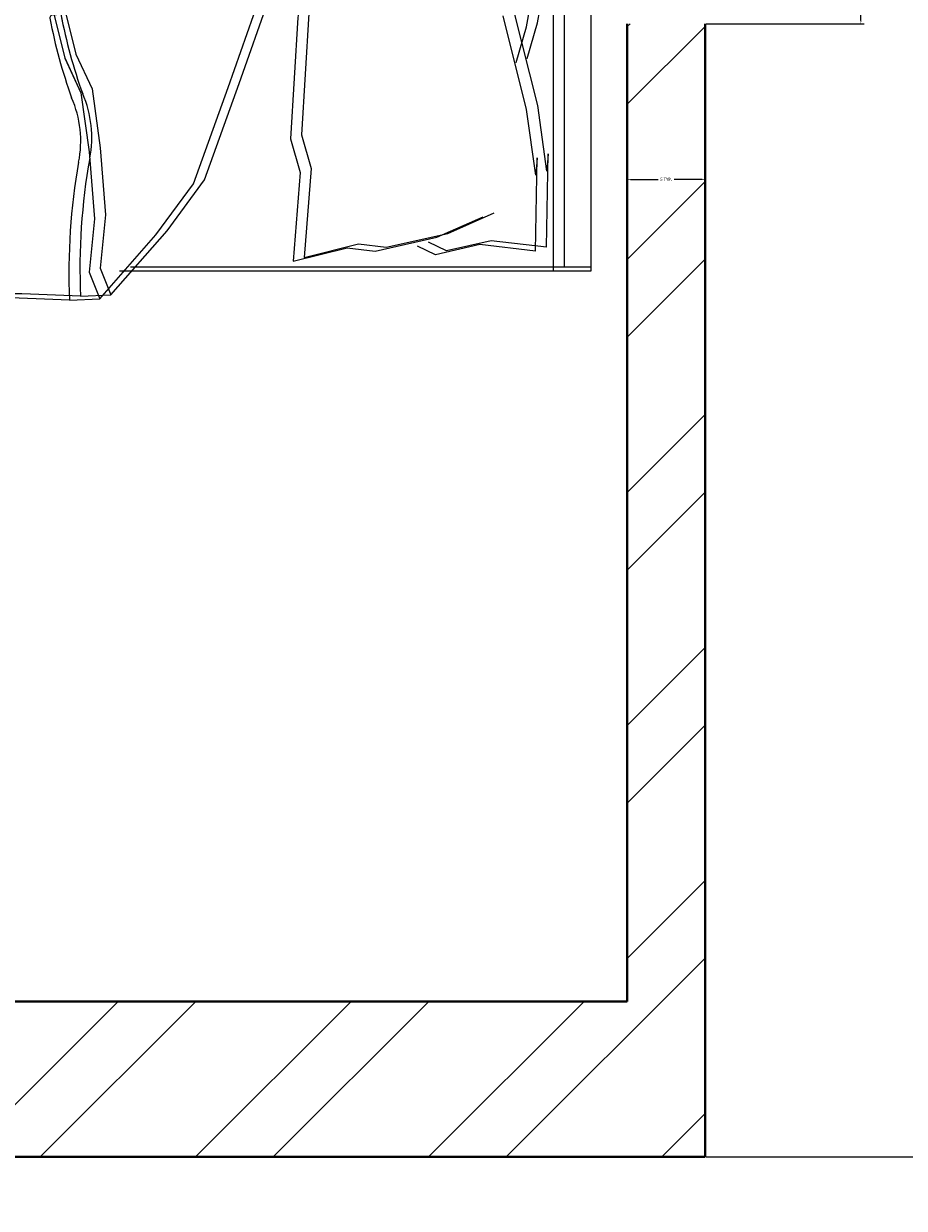
# Model space of a CAD drawing. Units: inches. Extents: x 1601 to 2297, y 1496 to 2631.
# Tile 19 of 57: x 2191 to 2242, y 1632 to 1701. Entities that reach past the tile are written whole.
import ezdxf

# ---------------------------------------------------------------- set-up
doc = ezdxf.new("R2010")
doc.units = ezdxf.units.IN
for name, color, linetype, lineweight in [('A-ANNO-DIMS', 2, 'Continuous', 18), ('A-FURN', 8, 'Continuous', 18), ('A-WALL', 7, 'Continuous', 40), ('A-WALL-PATT', 215, 'Continuous', 13)]:
    doc.layers.add(name, color=color, linetype=linetype, lineweight=lineweight)
doc.styles.get("Standard").update_dxf_attribs({"font": 'arial.ttf'})
doc.dimstyles.get("Standard").update_dxf_attribs({"dimtxt": 0.18, "dimasz": 0.18, "dimexe": 0.18, "dimexo": 0.0625, "dimgap": 0.09, "dimtad": 0, "dimtih": 1, "dimtoh": 1, "dimdec": 4, "dimzin": 0, "dimdsep": 46, "dimtxsty": 'Standard', "dimcen": 0.09, "dimadec": 0, "dimazin": 0, "dimtfac": 1, "dimtdec": 4, "dimtofl": 0, "dimtmove": 0, "dimatfit": 3, "dimfxl": 1, "dimtolj": 1, "dimtzin": 0, "dimarcsym": 0})

# ---------------------------------------------------------------- blocks, each defined once
blk = doc.blocks.new('BED-DOUBLE')
for p, q in [((27.746, 52.867), (24.495, 49.162)), ((27.746, 52.867), (24.495, 49.162)), ((27.746, 52.867), (24.495, 49.162)), ((27.746, 52.867), (24.495, 49.162)), ((28.385, 53.096), (25.135, 49.39)), ((28.385, 53.096), (25.135, 49.39)), ((28.385, 53.096), (25.135, 49.39)), ((28.385, 53.096), (25.135, 49.39)), ((29.49, 52.947), (27.746, 52.867, 3.871)), ((29.49, 52.947), (27.746, 52.867, 3.871)), ((29.49, 52.947), (27.746, 52.867, 3.871)), ((29.49, 52.947), (27.746, 52.867, 3.871)), ((28.365, 51.33), (27.746, 52.867)), ((28.365, 51.33), (27.746, 52.867)), ((28.365, 51.33), (27.746, 52.867)), ((28.365, 51.33), (27.746, 52.867)), ((30.13, 53.175), (28.385, 53.096, 3.871)), ((30.13, 53.175), (28.385, 53.096, 3.871)), ((30.13, 53.175), (28.385, 53.096, 3.871)), ((30.13, 53.175), (28.385, 53.096, 3.871)), ((29.004, 51.559), (28.385, 53.096)), ((29.004, 51.558), (28.385, 53.096)), ((29.004, 51.559), (28.385, 53.096)), ((29.004, 51.558), (28.385, 53.096)), ((0, 51.494), (0.639, 51.493)), ((0, 3.475), (0, 51.494)), ((0, 51.494), (0.639, 51.493)), ((0, 3.475), (0, 51.494)), ((0.639, 51.494), (27.249, 51.494)), ((0.639, 51.494), (27.249, 51.494)), ((0.639, 51.493), (27.249, 51.493)), ((0.639, 51.493), (27.249, 51.493)), ((2.173, 3.703), (2.173, 51.494)), ((2.173, 3.703), (2.173, 51.494)), ((2.173, 3.703), (2.173, 51.493)), ((2.173, 3.703), (2.173, 51.493)), ((28.695, 48.461), (29.004, 51.559)), ((28.695, 48.461), (29.004, 51.559)), ((28.695, 48.461), (29.004, 51.558)), ((28.695, 48.461), (29.004, 51.558)), ((0, 51.265), (26.61, 51.265)), ((0, 51.265), (26.61, 51.265)), ((0, 51.265), (26.61, 51.265)), ((0, 51.265), (26.61, 51.265)), ((1.533, 3.475), (1.533, 51.265)), ((1.533, 3.475), (1.533, 51.265)), ((1.533, 3.475), (1.533, 51.265)), ((1.533, 3.475), (1.533, 51.265)), ((16.573, 50.698), (13.434, 49.923)), ((16.573, 50.698), (13.434, 49.922)), ((16.573, 50.698), (13.434, 49.923)), ((16.573, 50.698), (13.434, 49.922)), ((17.212, 50.926), (14.073, 50.151)), ((17.212, 50.926), (14.073, 50.151)), ((17.212, 50.926), (14.073, 50.151)), ((17.212, 50.926), (14.073, 50.151)), ((16.169, 45.566), (16.573, 50.698)), ((16.169, 45.566), (16.573, 50.698)), ((16.169, 45.566), (16.573, 50.698)), ((16.169, 45.566), (16.573, 50.698)), ((16.808, 45.795), (17.212, 50.926)), ((16.808, 45.794), (17.212, 50.926)), ((16.808, 45.795), (17.212, 50.926)), ((16.808, 45.794), (17.212, 50.926)), ((28.055, 48.233), (28.365, 51.33)), ((28.055, 48.233), (28.365, 51.33)), ((28.055, 48.233), (28.365, 51.33)), ((28.055, 48.233), (28.365, 51.33)), ((2.557, 50.112), (2.46, 44.709)), ((2.557, 50.112), (2.46, 44.709)), ((2.557, 50.111), (2.46, 44.709)), ((2.557, 50.111), (2.46, 44.709)), ((2.557, 50.112), (5.768, 49.733)), ((2.557, 50.112), (5.768, 49.733)), ((2.557, 50.111), (5.768, 49.733)), ((2.557, 50.111), (5.768, 49.733)), ((3.196, 50.34), (3.099, 44.938)), ((3.196, 50.34), (3.099, 44.938)), ((3.196, 50.34), (3.099, 44.938)), ((3.196, 50.34), (3.099, 44.938)), ((3.196, 50.34), (6.407, 49.961)), ((3.196, 50.34), (6.407, 49.961)), ((3.196, 50.34), (6.407, 49.961)), ((3.196, 50.34), (6.407, 49.961)), ((5.768, 49.733), (8.338, 50.328)), ((5.768, 49.733), (8.338, 50.328)), ((5.768, 49.733), (8.338, 50.328)), ((5.768, 49.733), (8.338, 50.328)), ((6.407, 49.961), (8.977, 50.557)), ((6.407, 49.961), (8.977, 50.557)), ((6.407, 49.961), (8.977, 50.556)), ((6.407, 49.961), (8.977, 50.556)), ((11.829, 50.112), (8.257, 49.309)), ((11.829, 50.112), (8.257, 49.309)), ((11.829, 50.112), (8.257, 49.309)), ((11.829, 50.112), (8.257, 49.309)), ((8.338, 50.328), (9.384, 49.814)), ((8.338, 50.328), (9.384, 49.814)), ((8.338, 50.328), (9.384, 49.814)), ((8.338, 50.328), (9.384, 49.814)), ((12.468, 50.34), (8.896, 49.538)), ((12.468, 50.34), (8.896, 49.537)), ((12.468, 50.34), (8.896, 49.538)), ((12.468, 50.34), (8.896, 49.537)), ((8.977, 50.557), (10.024, 50.043)), ((8.977, 50.557), (10.024, 50.043)), ((8.977, 50.556), (10.024, 50.042)), ((8.977, 50.556), (10.024, 50.042)), ((13.434, 49.923), (11.829, 50.112)), ((13.434, 49.922), (11.829, 50.112)), ((13.434, 49.923), (11.829, 50.112)), ((13.434, 49.922), (11.829, 50.112)), ((14.073, 50.151), (12.468, 50.34)), ((14.073, 50.151), (12.468, 50.34)), ((14.073, 50.151), (12.468, 50.34)), ((14.073, 50.151), (12.468, 50.34)), ((8.896, 49.538), (6.218, 48.356)), ((8.896, 49.538), (6.218, 48.356)), ((8.896, 49.537), (6.218, 48.356)), ((8.896, 49.537), (6.218, 48.356)), ((25.135, 49.39), (22.968, 46.448)), ((25.135, 49.39), (22.968, 46.448)), ((25.135, 49.39), (22.968, 46.448)), ((25.135, 49.39), (22.968, 46.448)), ((8.257, 49.309), (5.578, 48.128)), ((8.257, 49.309), (5.578, 48.128)), ((8.257, 49.309), (5.578, 48.128)), ((8.257, 49.309), (5.578, 48.128)), ((24.495, 49.162), (22.329, 46.219)), ((24.495, 49.162), (22.329, 46.219)), ((24.495, 49.162), (22.329, 46.219)), ((24.495, 49.162), (22.329, 46.219)), ((28.365, 44.361), (28.055, 48.233)), ((28.365, 44.361), (28.055, 48.233)), ((28.365, 44.361), (28.055, 48.233)), ((28.365, 44.361), (28.055, 48.233)), ((29.004, 44.589), (28.695, 48.461)), ((29.004, 44.589), (28.695, 48.461)), ((29.004, 44.589), (28.695, 48.461)), ((29.004, 44.589), (28.695, 48.461)), ((3.099, 44.938), (3.181, 45.941)), ((3.099, 44.938), (3.181, 45.941)), ((3.099, 44.938), (3.181, 45.94)), ((3.099, 44.938), (3.181, 45.94)), ((3.181, 45.941), (3.709, 42.143)), ((3.181, 45.941), (3.709, 42.143)), ((3.181, 45.94), (3.709, 42.142)), ((3.181, 45.94), (3.709, 42.142)), ((22.329, 46.219), (20.316, 40.644)), ((22.329, 46.219), (20.316, 40.644)), ((22.329, 46.219), (20.317, 40.644)), ((22.329, 46.219), (20.317, 40.644)), ((22.968, 46.448), (20.956, 40.872)), ((22.968, 46.448), (20.956, 40.872)), ((22.968, 46.448), (20.956, 40.872)), ((22.968, 46.448), (20.956, 40.872)), ((2.46, 44.709), (2.542, 45.712)), ((2.46, 44.709), (2.542, 45.712)), ((2.46, 44.709), (2.542, 45.712)), ((2.46, 44.709), (2.542, 45.712)), ((2.542, 45.712), (3.069, 41.914)), ((2.542, 45.712), (3.069, 41.914)), ((2.542, 45.712), (3.069, 41.914)), ((2.542, 45.712), (3.069, 41.914)), ((16.726, 43.606), (16.169, 45.566)), ((16.726, 43.606), (16.169, 45.566)), ((16.726, 43.606), (16.169, 45.566)), ((16.726, 43.606), (16.169, 45.566)), ((17.365, 43.834), (16.808, 45.795)), ((17.365, 43.834), (16.808, 45.795)), ((17.365, 43.834), (16.808, 45.794)), ((17.365, 43.834), (16.808, 45.794)), ((29.468, 41.182), (29.004, 44.589)), ((29.469, 41.182), (29.004, 44.589)), ((29.468, 41.182), (29.004, 44.589)), ((29.469, 41.182), (29.004, 44.589)), ((28.829, 40.954), (28.365, 44.361)), ((28.829, 40.953), (28.365, 44.361)), ((28.829, 40.954), (28.365, 44.361)), ((28.829, 40.953), (28.365, 44.361)), ((16.295, 36.596), (16.726, 43.606)), ((16.295, 36.596), (16.726, 43.606)), ((16.295, 36.596), (16.726, 43.606)), ((16.295, 36.596), (16.726, 43.606)), ((16.934, 36.824), (17.365, 43.834)), ((16.934, 36.824), (17.365, 43.834)), ((16.934, 36.824), (17.365, 43.834)), ((16.934, 36.824), (17.365, 43.834)), ((3.069, 41.914), (4.422, 36.495)), ((3.069, 41.914), (4.422, 36.495)), ((3.069, 41.914), (4.422, 36.495)), ((3.069, 41.914), (4.422, 36.495)), ((3.709, 42.143), (5.061, 36.723)), ((3.709, 42.143), (5.061, 36.723)), ((3.709, 42.142), (5.061, 36.723)), ((3.709, 42.142), (5.061, 36.723)), ((30.397, 39.169), (29.468, 41.182)), ((30.397, 39.169), (29.468, 41.182)), ((30.397, 39.168), (29.469, 41.182)), ((30.397, 39.168), (29.469, 41.182)), ((20.316, 40.644), (17.383, 32.306)), ((20.317, 40.644), (17.383, 32.306)), ((20.316, 40.644), (17.383, 32.306)), ((20.317, 40.644), (17.383, 32.306)), ((20.956, 40.872), (18.022, 32.534)), ((20.956, 40.872), (18.022, 32.534)), ((20.956, 40.872), (18.022, 32.534)), ((20.956, 40.872), (18.022, 32.534)), ((29.758, 38.94), (28.829, 40.954)), ((29.758, 38.94), (28.829, 40.954)), ((29.758, 38.94), (28.829, 40.953)), ((29.758, 38.94), (28.829, 40.953)), ((79.884, 15.292), (79.884, 39.905)), ((79.884, 15.291), (79.884, 39.905)), ((79.884, 15.292), (79.884, 39.905)), ((79.884, 15.291), (79.884, 39.905)), ((3.673, 39.2), (3.078, 37.135)), ((3.673, 39.2), (3.078, 37.135)), ((3.673, 39.2), (3.078, 37.135)), ((3.673, 39.2), (3.078, 37.135)), ((4.313, 39.428), (3.717, 37.363)), ((4.313, 39.428), (3.717, 37.363)), ((4.313, 39.428), (3.718, 37.363)), ((4.313, 39.428), (3.718, 37.363)), ((31.016, 36.691), (30.397, 39.169)), ((31.016, 36.691), (30.397, 39.169)), ((31.016, 36.691), (30.397, 39.168)), ((31.016, 36.691), (30.397, 39.168)), ((79.245, 15.063), (79.245, 39.677)), ((79.245, 15.063), (79.245, 39.677)), ((79.245, 15.063), (79.245, 39.677)), ((79.245, 15.063), (79.245, 39.677)), ((30.377, 36.462), (29.758, 38.94)), ((30.377, 36.462), (29.758, 38.94)), ((30.377, 36.462), (29.758, 38.94)), ((30.377, 36.462), (29.758, 38.94)), ((3.078, 37.135), (2.537, 34.204)), ((3.078, 37.135), (2.537, 34.204)), ((3.078, 37.135), (2.537, 34.204)), ((3.078, 37.135), (2.537, 34.204)), ((3.717, 37.363), (3.176, 34.433)), ((3.718, 37.363), (3.176, 34.433)), ((3.717, 37.363), (3.176, 34.433)), ((3.718, 37.363), (3.176, 34.433)), ((15.628, 32.564), (16.295, 36.596)), ((15.628, 32.564), (16.295, 36.596)), ((15.628, 32.564), (16.295, 36.596)), ((15.628, 32.564), (16.295, 36.596)), ((16.268, 32.792), (16.934, 36.824)), ((16.268, 32.792), (16.934, 36.824)), ((16.268, 32.792), (16.934, 36.824)), ((16.268, 32.792), (16.934, 36.824)), ((24.516, 34.677), (29.004, 36.381)), ((24.516, 34.677), (29.004, 36.381)), ((24.516, 34.677), (29.004, 36.381)), ((24.516, 34.677), (29.004, 36.381)), ((28.365, 36.153), (30.377, 36.462)), ((28.365, 36.152), (30.377, 36.462)), ((28.365, 36.153), (30.377, 36.462)), ((28.365, 36.152), (30.377, 36.462)), ((29.004, 36.381), (31.016, 36.691)), ((29.004, 36.381), (31.016, 36.691)), ((29.004, 36.381), (31.016, 36.691)), ((29.004, 36.381), (31.016, 36.691)), ((23.876, 34.449), (28.365, 36.153)), ((23.876, 34.449), (28.365, 36.153)), ((23.876, 34.449), (28.365, 36.152)), ((23.876, 34.449), (28.365, 36.152)), ((3.176, 34.433), (3.196, 34.112)), ((3.176, 34.433), (3.196, 34.112)), ((3.176, 34.433), (3.196, 34.112)), ((3.176, 34.433), (3.196, 34.112)), ((17.383, 30.259), (23.876, 34.449)), ((17.383, 30.259), (23.876, 34.449)), ((17.383, 30.259), (23.876, 34.449)), ((17.383, 30.259), (23.876, 34.449)), ((18.022, 30.487), (24.516, 34.677)), ((18.022, 30.487), (24.516, 34.677)), ((18.022, 30.487), (24.516, 34.677)), ((18.022, 30.487), (24.516, 34.677)), ((2.537, 34.204), (2.557, 33.883)), ((2.537, 34.204), (2.557, 33.883)), ((2.537, 34.204), (2.557, 33.883)), ((2.537, 34.204), (2.557, 33.883)), ((2.557, 33.883), (2.979, 29.456)), ((2.557, 33.883), (2.979, 29.455)), ((2.557, 33.883), (2.979, 29.456)), ((2.557, 33.883), (2.979, 29.455)), ((3.196, 34.112), (3.618, 29.684)), ((3.196, 34.112), (3.618, 29.684)), ((3.196, 34.112), (3.618, 29.684)), ((3.196, 34.112), (3.618, 29.684)), ((16.739, 30.75), (15.454, 33.821)), ((16.739, 30.75), (15.454, 33.821)), ((16.739, 30.75), (15.454, 33.82)), ((16.739, 30.75), (15.454, 33.82)), ((17.379, 30.978), (16.094, 34.049)), ((17.379, 30.978), (16.094, 34.049)), ((17.379, 30.978), (16.094, 34.049)), ((17.379, 30.978), (16.094, 34.049)), ((17.532, 28.526), (17.379, 30.978)), ((17.532, 28.525), (17.379, 30.978)), ((17.532, 28.526), (17.379, 30.978)), ((17.532, 28.525), (17.379, 30.978)), ((16.893, 28.297), (16.739, 30.75)), ((16.893, 28.297), (16.739, 30.75)), ((16.893, 28.297), (16.739, 30.75)), ((16.893, 28.297), (16.739, 30.75)), ((2.979, 29.456), (2.492, 27.977)), ((2.979, 29.456), (2.492, 27.977)), ((2.979, 29.455), (2.492, 27.976)), ((2.979, 29.455), (2.492, 27.976)), ((3.618, 29.684), (3.131, 28.205)), ((3.618, 29.684), (3.131, 28.205)), ((3.618, 29.684), (3.131, 28.205)), ((3.618, 29.684), (3.131, 28.205)), ((3.131, 28.205), (8.506, 27.962)), ((3.131, 28.205), (8.506, 27.961)), ((3.131, 28.205), (8.506, 27.962)), ((3.131, 28.205), (8.506, 27.961)), ((12.377, 27.436), (14.216, 28.13)), ((12.377, 27.436), (14.217, 28.13)), ((12.377, 27.436), (14.216, 28.13)), ((12.377, 27.436), (14.217, 28.13)), ((13.016, 27.664), (14.856, 28.359)), ((13.016, 27.664), (14.856, 28.359)), ((13.016, 27.664), (14.856, 28.358)), ((13.016, 27.664), (14.856, 28.358)), ((14.216, 28.13), (16.893, 28.297)), ((14.216, 28.13), (16.893, 28.297)), ((14.217, 28.13), (16.893, 28.297)), ((14.217, 28.13), (16.893, 28.297)), ((14.856, 28.359), (17.532, 28.526)), ((14.856, 28.359), (17.532, 28.526)), ((14.856, 28.358), (17.532, 28.525)), ((14.856, 28.358), (17.532, 28.525)), ((2.492, 27.977), (7.867, 27.733)), ((2.492, 27.977), (7.867, 27.733)), ((2.492, 27.976), (7.867, 27.733)), ((2.492, 27.976), (7.867, 27.733)), ((7.867, 27.733), (11.078, 27.355)), ((7.867, 27.733), (11.078, 27.354)), ((7.867, 27.733), (11.078, 27.355)), ((7.867, 27.733), (11.078, 27.354)), ((8.506, 27.962), (11.717, 27.583)), ((8.506, 27.962), (11.717, 27.583)), ((8.506, 27.961), (11.717, 27.583)), ((8.506, 27.961), (11.717, 27.583)), ((11.078, 27.355), (12.377, 27.436)), ((11.078, 27.354), (12.377, 27.436)), ((11.078, 27.355), (12.377, 27.436)), ((11.078, 27.354), (12.377, 27.436)), ((11.717, 27.583), (13.016, 27.664)), ((11.717, 27.583), (13.016, 27.664)), ((11.717, 27.583), (13.016, 27.664)), ((11.717, 27.583), (13.016, 27.664)), ((2.509, 26.211), (7.859, 26.789)), ((2.509, 26.21), (7.859, 26.789)), ((2.509, 26.211), (7.859, 26.789)), ((2.509, 26.21), (7.859, 26.789)), ((7.22, 26.561), (10.401, 27.139)), ((7.22, 26.56), (10.401, 27.139)), ((7.22, 26.561), (10.401, 27.139)), ((7.22, 26.56), (10.401, 27.139)), ((7.859, 26.789), (11.04, 27.367)), ((7.859, 26.789), (11.04, 27.367)), ((7.859, 26.789), (11.04, 27.367)), ((7.859, 26.789), (11.04, 27.367)), ((10.401, 27.139), (11.702, 27.139)), ((10.401, 27.139), (11.702, 27.139)), ((10.401, 27.139), (11.702, 27.139)), ((10.401, 27.139), (11.702, 27.139)), ((11.04, 27.367), (12.341, 27.367)), ((11.04, 27.367), (12.341, 27.367)), ((11.04, 27.367), (12.341, 27.367)), ((11.04, 27.367), (12.341, 27.367)), ((11.702, 27.139), (13.582, 26.561)), ((11.702, 27.139), (13.582, 26.56)), ((11.702, 27.139), (13.582, 26.561)), ((11.702, 27.139), (13.582, 26.56)), ((12.341, 27.367), (14.221, 26.789)), ((12.341, 27.367), (14.221, 26.789)), ((12.341, 27.367), (14.221, 26.789)), ((12.341, 27.367), (14.221, 26.789)), ((14.221, 26.789), (16.902, 26.789)), ((14.221, 26.789), (16.902, 26.789)), ((14.221, 26.789), (16.902, 26.789)), ((14.221, 26.789), (16.902, 26.789)), ((16.902, 26.789), (16.902, 24.332)), ((16.902, 26.789), (16.902, 24.331)), ((16.902, 26.789), (16.902, 24.332)), ((16.902, 26.789), (16.902, 24.331)), ((1.87, 25.982), (7.22, 26.561)), ((1.87, 25.982), (7.22, 26.561)), ((1.87, 25.982), (7.22, 26.56)), ((1.87, 25.982), (7.22, 26.56)), ((3.088, 24.765), (2.509, 26.211)), ((3.088, 24.765), (2.509, 26.211)), ((3.088, 24.765), (2.509, 26.21)), ((3.088, 24.765), (2.509, 26.21)), ((13.582, 26.561), (16.263, 26.561)), ((13.582, 26.561), (16.263, 26.561)), ((13.582, 26.56), (16.263, 26.56)), ((13.582, 26.56), (16.263, 26.56)), ((16.263, 26.561), (16.263, 24.103)), ((16.263, 26.561), (16.263, 24.103)), ((16.263, 26.56), (16.263, 24.103)), ((16.263, 26.56), (16.263, 24.103)), ((2.448, 24.537), (1.87, 25.982)), ((2.448, 24.537), (1.87, 25.982)), ((2.448, 24.537), (1.87, 25.982)), ((2.448, 24.537), (1.87, 25.982)), ((2.943, 20.32), (3.088, 24.765)), ((2.943, 20.319), (3.088, 24.765)), ((2.943, 20.32), (3.088, 24.765)), ((2.943, 20.319), (3.088, 24.765)), ((16.808, 19.612), (17.212, 24.744)), ((16.808, 19.612), (17.212, 24.744)), ((16.808, 19.612), (17.212, 24.744)), ((16.808, 19.612), (17.212, 24.744)), ((2.304, 20.091), (2.448, 24.537)), ((2.304, 20.091), (2.448, 24.537)), ((2.304, 20.091), (2.448, 24.537)), ((2.304, 20.091), (2.448, 24.537)), ((16.263, 24.103), (15.172, 20.959)), ((16.263, 24.103), (15.172, 20.958)), ((16.263, 24.103), (15.172, 20.959)), ((16.263, 24.103), (15.172, 20.958)), ((16.902, 24.332), (15.811, 21.187)), ((16.902, 24.332), (15.811, 21.187)), ((16.902, 24.331), (15.811, 21.187)), ((16.902, 24.331), (15.811, 21.187)), ((16.169, 19.384), (16.573, 24.516)), ((16.169, 19.384), (16.573, 24.516)), ((16.169, 19.383), (16.573, 24.515)), ((16.169, 19.383), (16.573, 24.515)), ((2.304, 19.77), (2.304, 20.091)), ((2.304, 19.769), (2.304, 20.091)), ((2.304, 19.77), (2.304, 20.091)), ((2.304, 19.769), (2.304, 20.091)), ((2.943, 19.998), (2.943, 20.32)), ((2.943, 19.998), (2.943, 20.32)), ((2.943, 19.998), (2.943, 20.319)), ((2.943, 19.998), (2.943, 20.319)), ((3.666, 17.107), (2.943, 19.998)), ((3.666, 17.107), (2.943, 19.998)), ((3.666, 17.107), (2.943, 19.998)), ((3.666, 17.107), (2.943, 19.998)), ((3.027, 16.878), (2.304, 19.77)), ((3.027, 16.878), (2.304, 19.77)), ((3.027, 16.878), (2.304, 19.769)), ((3.027, 16.878), (2.304, 19.769)), ((16.726, 17.423), (16.169, 19.384)), ((16.726, 17.423), (16.169, 19.384)), ((16.726, 17.423), (16.169, 19.383)), ((16.726, 17.423), (16.169, 19.383)), ((17.365, 17.652), (16.808, 19.612)), ((17.365, 17.651), (16.808, 19.612)), ((17.365, 17.652), (16.808, 19.612)), ((17.365, 17.651), (16.808, 19.612)), ((3.955, 12.336), (4.967, 17.83)), ((3.955, 12.336), (4.967, 17.83)), ((3.955, 12.336), (4.967, 17.829)), ((3.955, 12.336), (4.967, 17.829)), ((3.316, 12.108), (4.328, 17.601)), ((3.316, 12.108), (4.328, 17.601)), ((3.316, 12.108), (4.328, 17.601)), ((3.316, 12.108), (4.328, 17.601)), ((16.295, 10.413), (16.726, 17.423)), ((16.295, 10.413), (16.726, 17.423)), ((16.295, 10.413), (16.726, 17.423)), ((16.295, 10.413), (16.726, 17.423)), ((16.934, 10.642), (17.365, 17.652)), ((16.934, 10.642), (17.365, 17.652)), ((16.934, 10.642), (17.365, 17.651)), ((16.934, 10.642), (17.365, 17.651)), ((3.75, 14.855), (3.027, 16.878)), ((3.75, 14.854), (3.027, 16.878)), ((3.75, 14.855), (3.027, 16.878)), ((3.75, 14.854), (3.027, 16.878)), ((4.389, 15.083), (3.666, 17.107)), ((4.389, 15.083), (3.666, 17.107)), ((4.389, 15.083), (3.666, 17.107)), ((4.389, 15.083), (3.666, 17.107)), ((3.666, 8.513), (3.955, 12.336)), ((3.666, 8.513), (3.955, 12.336)), ((3.666, 8.513), (3.955, 12.336)), ((3.666, 8.513), (3.955, 12.336)), ((3.027, 8.285), (3.316, 12.108)), ((3.027, 8.284), (3.316, 12.108)), ((3.027, 8.285), (3.316, 12.108)), ((3.027, 8.284), (3.316, 12.108)), ((15.628, 6.382), (16.295, 10.413)), ((15.628, 6.381), (16.295, 10.413)), ((15.628, 6.382), (16.295, 10.413)), ((15.628, 6.381), (16.295, 10.413)), ((16.268, 6.61), (16.934, 10.642)), ((16.268, 6.61), (16.934, 10.642)), ((16.268, 6.61), (16.934, 10.642)), ((16.268, 6.61), (16.934, 10.642)), ((16.295, 10.413), (16.618, 9.28)), ((16.295, 10.413), (16.618, 9.28)), ((16.295, 10.413), (16.618, 9.28)), ((16.295, 10.413), (16.618, 9.28)), ((16.934, 10.642), (17.257, 9.509)), ((16.934, 10.642), (17.257, 9.508)), ((16.934, 10.642), (17.257, 9.509)), ((16.934, 10.642), (17.257, 9.508)), ((16.618, 9.28), (17.341, 4.184)), ((16.618, 9.28), (17.341, 4.183)), ((16.618, 9.28), (17.341, 4.184)), ((16.618, 9.28), (17.341, 4.183)), ((17.257, 9.509), (17.98, 4.412)), ((17.257, 9.509), (17.98, 4.412)), ((17.257, 9.508), (17.98, 4.412)), ((17.257, 9.508), (17.98, 4.412)), ((3.009, 8.179), (3.027, 8.285)), ((3.009, 8.179), (3.027, 8.285)), ((3.009, 8.179), (3.027, 8.284)), ((3.009, 8.179), (3.027, 8.284)), ((3.648, 8.408), (3.666, 8.513)), ((3.648, 8.407), (3.666, 8.513)), ((3.648, 8.408), (3.666, 8.513)), ((3.648, 8.407), (3.666, 8.513)), ((3.977, 4.127), (3.648, 8.408)), ((3.977, 4.127), (3.648, 8.408)), ((3.977, 4.127), (3.648, 8.407)), ((3.977, 4.127), (3.648, 8.407)), ((3.338, 3.898), (3.009, 8.179)), ((3.338, 3.898), (3.009, 8.179)), ((3.338, 3.898), (3.009, 8.179)), ((3.338, 3.898), (3.009, 8.179)), ((9.594, 5.279), (6.847, 6.291)), ((9.594, 5.279), (6.847, 6.291)), ((9.594, 5.279), (6.847, 6.291)), ((9.594, 5.279), (6.847, 6.291)), ((8.955, 5.051), (6.208, 6.063)), ((8.955, 5.051), (6.208, 6.063)), ((8.955, 5.051), (6.208, 6.063)), ((8.955, 5.051), (6.208, 6.063)), ((12.57, 4.473), (8.955, 5.051)), ((12.57, 4.472), (8.955, 5.051)), ((12.57, 4.473), (8.955, 5.051)), ((12.57, 4.472), (8.955, 5.051)), ((13.209, 4.701), (9.594, 5.279)), ((13.209, 4.701), (9.594, 5.279)), ((13.209, 4.701), (9.594, 5.279)), ((13.209, 4.701), (9.594, 5.279)), ((9.739, 4.267), (10.751, 4.846)), ((9.739, 4.267), (10.751, 4.846)), ((9.739, 4.267), (10.751, 4.845)), ((9.739, 4.267), (10.751, 4.845)), ((14.799, 4.99), (13.209, 4.701)), ((14.799, 4.99), (13.209, 4.701)), ((14.799, 4.99), (13.209, 4.701)), ((14.799, 4.99), (13.209, 4.701)), ((17.98, 4.412), (14.799, 4.99)), ((17.98, 4.412), (14.799, 4.99)), ((17.98, 4.412), (14.799, 4.99)), ((17.98, 4.412), (14.799, 4.99)), ((3.316, 3.894), (6.497, 4.473)), ((3.316, 3.894), (6.497, 4.473)), ((3.316, 3.894), (6.497, 4.472)), ((3.316, 3.894), (6.497, 4.472)), ((3.955, 4.123), (7.136, 4.701)), ((3.955, 4.123), (7.136, 4.701)), ((3.955, 4.123), (7.136, 4.701)), ((3.955, 4.123), (7.136, 4.701)), ((6.497, 4.473), (9.099, 4.039)), ((6.497, 4.473), (9.099, 4.039)), ((6.497, 4.472), (9.099, 4.039)), ((6.497, 4.472), (9.099, 4.039)), ((7.136, 4.701), (9.739, 4.267)), ((7.136, 4.701), (9.739, 4.267)), ((7.136, 4.701), (9.739, 4.267)), ((7.136, 4.701), (9.739, 4.267)), ((9.099, 4.039), (10.112, 4.617)), ((9.099, 4.039), (10.112, 4.617)), ((9.099, 4.039), (10.112, 4.617)), ((9.099, 4.039), (10.112, 4.617)), ((14.16, 4.762), (12.57, 4.473)), ((14.16, 4.762), (12.57, 4.472)), ((14.16, 4.762), (12.57, 4.473)), ((14.16, 4.762), (12.57, 4.472)), ((17.341, 4.184), (14.16, 4.762)), ((17.341, 4.183), (14.16, 4.762)), ((17.341, 4.184), (14.16, 4.762)), ((17.341, 4.183), (14.16, 4.762)), ((18.11, 3.475), (0, 3.475)), ((18.11, 3.475), (0, 3.475)), ((18.11, 3.475), (0, 3.475)), ((18.11, 3.475), (0, 3.475)), ((18.75, 3.703), (0.639, 3.703)), ((18.75, 3.703), (0.639, 3.703)), ((18.75, 3.703), (0.639, 3.703)), ((18.75, 3.703), (0.639, 3.703))]:
    blk.add_line(p, q)
for centre, radius, start, end in [((68.666, 76.157), 23.065, 267.47136, 296.46809), ((68.666, 76.157), 23.065, 267.47136, 296.46809), ((68.666, 76.157), 23.065, 267.47136, 296.46809), ((68.666, 76.157), 23.065, 267.47136, 296.46809), ((69.306, 76.385), 23.065, 267.47136, 296.46809), ((69.306, 76.385), 23.065, 267.47136, 296.46809), ((69.306, 76.385), 23.065, 267.47136, 296.46809), ((69.306, 76.385), 23.065, 267.47136, 296.46809), ((78.87, 54.41), 1.102, 332.65876, 86.02002), ((78.87, 54.409), 1.102, 332.65876, 86.02002), ((78.87, 54.41), 1.102, 332.65876, 86.02002), ((78.87, 54.409), 1.102, 332.65876, 86.02002), ((79.509, 54.638), 1.102, 332.65876, 86.02002), ((79.509, 54.638), 1.102, 332.65876, 86.02002), ((79.509, 54.638), 1.102, 332.65876, 86.02002), ((79.509, 54.638), 1.102, 332.65876, 86.02002), ((212.916, 41.38), 133.04, 174.4998, 180.63509), ((212.916, 41.38), 133.04, 174.4998, 180.63509), ((212.916, 41.38), 133.04, 174.4998, 180.63509), ((212.916, 41.38), 133.04, 174.4998, 180.63509), ((212.276, 41.152), 133.04, 174.4998, 180.63509), ((212.277, 41.151), 133.04, 174.4998, 180.63509), ((212.276, 41.152), 133.04, 174.4998, 180.63509), ((212.277, 41.151), 133.04, 174.4998, 180.63509), ((-6.656, 51.327), 36.183, 349.87628, 2.56571), ((-6.656, 51.327), 36.183, 349.87628, 2.56571), ((-6.656, 51.327), 36.183, 349.87628, 2.56571), ((-6.656, 51.327), 36.183, 349.87628, 2.56571), ((36.315, 182.266), 129.499, 266.97912, 273.83645), ((36.315, 182.265), 129.499, 266.97912, 273.83645), ((36.315, 182.266), 129.499, 266.97912, 273.83645), ((36.315, 182.265), 129.499, 266.97912, 273.83645), ((-6.017, 51.555), 36.183, 349.87628, 2.56571), ((-6.017, 51.555), 36.183, 349.87628, 2.56571), ((-6.017, 51.555), 36.183, 349.87628, 2.56571), ((-6.017, 51.555), 36.183, 349.87628, 2.56571), ((36.954, 182.494), 129.499, 266.97912, 273.83645), ((36.954, 182.494), 129.499, 266.97912, 273.83645), ((36.954, 182.494), 129.499, 266.97912, 273.83645), ((36.954, 182.494), 129.499, 266.97912, 273.83645), ((67.821, -4508.744), 4561.858, 90.002168, 90.286887), ((67.821, -4508.744), 4561.858, 90.002168, 90.286887), ((67.821, -4508.744), 4561.858, 90.002168, 90.286887), ((67.821, -4508.744), 4561.858, 90.002168, 90.286887), ((68.461, -4508.515), 4561.858, 90.002168, 90.286887), ((68.461, -4508.515), 4561.858, 90.002168, 90.286887), ((68.461, -4508.516), 4561.858, 90.002168, 90.286887), ((68.461, -4508.516), 4561.858, 90.002168, 90.286887), ((35.066, 43.743), 6.224, 168.6608, 203.73842), ((35.066, 43.743), 6.224, 168.6608, 203.73842), ((35.066, 43.743), 6.224, 168.6608, 203.73842), ((35.066, 43.743), 6.224, 168.6608, 203.73842), ((35.705, 43.972), 6.224, 168.6608, 203.73842), ((35.705, 43.971), 6.224, 168.6608, 203.73842), ((35.705, 43.972), 6.224, 168.6608, 203.73842), ((35.705, 43.971), 6.224, 168.6608, 203.73842), ((1.482, 31.154), 29.654, 10.66171, 19.88058), ((1.482, 31.154), 29.654, 10.66171, 19.88058), ((1.482, 31.153), 29.654, 10.66171, 19.88058), ((1.482, 31.153), 29.654, 10.66171, 19.88058), ((2.121, 31.382), 29.654, 10.66171, 19.88058), ((2.121, 31.382), 29.654, 10.66171, 19.88058), ((2.121, 31.382), 29.654, 10.66171, 19.88058), ((2.121, 31.382), 29.654, 10.66171, 19.88058), ((156.955, 17.984), 129.02, 171.78449, 186.90062), ((156.955, 17.984), 129.02, 171.78449, 186.90062), ((156.955, 17.984), 129.02, 171.78449, 186.90062), ((156.955, 17.984), 129.02, 171.78449, 186.90062), ((30.439, 36.636), 0.185, 250.24637, 1.13765), ((30.439, 36.636), 0.185, 250.24637, 1.13765), ((30.439, 36.636), 0.185, 250.24637, 1.13765), ((30.439, 36.636), 0.185, 250.24637, 1.13765), ((31.079, 36.864), 0.185, 250.24637, 1.13765), ((31.079, 36.864), 0.185, 250.24637, 1.13765), ((31.079, 36.864), 0.185, 250.24637, 1.13765), ((31.079, 36.864), 0.185, 250.24637, 1.13765), ((156.316, 17.756), 129.02, 171.78449, 186.90062), ((156.316, 17.755), 129.02, 171.78449, 186.90062), ((156.316, 17.756), 129.02, 171.78449, 186.90062), ((156.316, 17.755), 129.02, 171.78449, 186.90062), ((182.052, 21.359), 164.969, 176.08655, 186.78213), ((182.052, 21.359), 164.969, 176.08655, 186.78213), ((182.052, 21.358), 164.969, 176.08655, 186.78213), ((182.052, 21.358), 164.969, 176.08655, 186.78213), ((182.692, 21.587), 164.969, 176.08655, 186.78213), ((182.692, 21.587), 164.969, 176.08655, 186.78213), ((182.692, 21.587), 164.969, 176.08655, 186.78213), ((182.692, 21.587), 164.969, 176.08655, 186.78213), ((-23.712, -17.222), 106.459, 13.38322, 17.70533), ((-23.712, -17.222), 106.459, 13.38322, 17.70533), ((-23.712, -17.222), 106.459, 13.38322, 17.70533), ((-23.712, -17.222), 106.459, 13.38322, 17.70533), ((-23.073, -16.994), 106.459, 13.38322, 17.70533), ((-23.073, -16.994), 106.459, 13.38322, 17.70533), ((-23.073, -16.994), 106.459, 13.38322, 17.70533), ((-23.073, -16.994), 106.459, 13.38322, 17.70533), ((201.476, 21.655), 121.759, 182.99578, 189.40907), ((201.476, 21.655), 121.759, 182.99578, 189.40907), ((201.476, 21.655), 121.759, 182.99578, 189.40907), ((201.476, 21.655), 121.759, 182.99578, 189.40907), ((200.837, 21.427), 121.759, 182.99578, 189.40907), ((200.837, 21.426), 121.759, 182.99578, 189.40907), ((200.837, 21.427), 121.759, 182.99578, 189.40907), ((200.837, 21.426), 121.759, 182.99578, 189.40907), ((31.174, -167.308), 170.11, 88.4762, 91.00819), ((31.174, -167.308), 170.11, 88.4762, 91.00819), ((31.174, -167.308), 170.11, 88.4762, 91.00819), ((31.174, -167.308), 170.11, 88.4762, 91.00819), ((31.813, -167.079), 170.11, 88.4762, 91.00819), ((31.813, -167.08), 170.11, 88.4762, 91.00819), ((31.813, -167.079), 170.11, 88.4762, 91.00819), ((31.813, -167.08), 170.11, 88.4762, 91.00819), ((50.614, 484.822), 482.31, 268.22771, 271.71854), ((50.614, 484.822), 482.31, 268.22771, 271.71854), ((50.614, 484.822), 482.31, 268.22771, 271.71854), ((50.614, 484.822), 482.31, 268.22771, 271.71854), ((51.253, 485.051), 482.31, 268.22771, 271.71854), ((51.253, 485.05), 482.31, 268.22771, 271.71854), ((51.253, 485.051), 482.31, 268.22771, 271.71854), ((51.253, 485.05), 482.31, 268.22771, 271.71854), ((65.154, -26.671), 29.634, 76.06484, 88.91125), ((65.154, -26.672), 29.634, 76.06484, 88.91125), ((65.154, -26.671), 29.634, 76.06484, 88.91125), ((65.154, -26.672), 29.634, 76.06484, 88.91125), ((20.096, 85.162), 83.306, 268.72178, 275.60397), ((20.096, 85.161), 83.306, 268.72178, 275.60397), ((20.096, 85.162), 83.306, 268.72178, 275.60397), ((20.096, 85.161), 83.306, 268.72178, 275.60397), ((20.735, 85.39), 83.306, 268.72178, 275.60397), ((20.735, 85.39), 83.306, 268.72178, 275.60397), ((20.736, 85.39), 83.306, 268.72178, 275.60397), ((20.736, 85.39), 83.306, 268.72178, 275.60397), ((64.515, -26.9), 29.634, 76.06484, 88.91125), ((64.515, -26.9), 29.634, 76.06484, 88.91125), ((64.515, -26.9), 29.634, 76.06484, 88.91125), ((64.515, -26.9), 29.634, 76.06484, 88.91125), ((70.915, -21.431), 23.562, 67.97508, 86.652), ((70.915, -21.432), 23.562, 67.97508, 86.652), ((70.915, -21.431), 23.562, 67.97508, 86.652), ((70.915, -21.432), 23.562, 67.97508, 86.652), ((70.276, -21.66), 23.562, 67.97508, 86.652), ((70.276, -21.66), 23.562, 67.97508, 86.652), ((70.276, -21.66), 23.562, 67.97508, 86.652), ((70.276, -21.66), 23.562, 67.97508, 86.652), ((79.718, 1.087), 1.089, 236.17358, 23.47814), ((79.718, 1.087), 1.089, 236.17358, 23.47814), ((79.718, 1.087), 1.089, 236.17358, 23.47814), ((79.718, 1.087), 1.089, 236.17358, 23.47814), ((80.357, 1.316), 1.089, 236.17358, 23.47814), ((80.357, 1.316), 1.089, 236.17358, 23.47814), ((80.357, 1.315), 1.089, 236.17358, 23.47814), ((80.357, 1.315), 1.089, 236.17358, 23.47814)]:
    blk.add_arc(centre, radius, start, end)
blk = doc.blocks.new('*D24')
at = {"layer": 'A-ANNO-DIMS', "color": 0, "lineweight": -2, "transparency": 16777216}
for p, q in [((2230.6, 1760.856), (2239.717, 1760.856)), ((2239.537, 1760.676), (2239.537, 1731.039)), ((2239.537, 1701.036), (2239.537, 1730.673)), ((2230.6, 1700.856), (2239.717, 1700.856))]:
    blk.add_line(p, q, dxfattribs=at)
at = {"layer": 'A-ANNO-DIMS', "color": 0, "transparency": 16777216}
for points in [[(2239.507, 1760.676), (2239.567, 1760.676), (2239.537, 1760.856)], [(2239.507, 1701.036), (2239.567, 1701.036), (2239.537, 1700.856)]]:
    blk.add_solid(points, dxfattribs=at)
at = {"layer": 'Defpoints', "color": 0, "transparency": 16777216}
for p in [(2230.537, 1760.856), (2239.537, 1760.856), (2230.537, 1700.856)]:
    blk.add_point(p, dxfattribs=at)
at = {"layer": 'A-ANNO-DIMS', "color": 0, "transparency": 16777216, "insert": (2239.537, 1730.856), "char_height": 0.18, "attachment_point": 5}
blk.add_mtext('\\A1;WINDOW 60 TYP.', dxfattribs=at)
blk = doc.blocks.new('*D25')
at = {"layer": 'A-ANNO-DIMS', "color": 0, "lineweight": -2, "transparency": 16777216}
for p, q in [((2226.037, 1700.794), (2226.037, 1691.676)), ((2230.537, 1700.794), (2230.537, 1691.676)), ((2226.217, 1691.856), (2227.829, 1691.856)), ((2230.357, 1691.856), (2228.745, 1691.856))]:
    blk.add_line(p, q, dxfattribs=at)
at = {"layer": 'A-ANNO-DIMS', "color": 0, "transparency": 16777216}
for points in [[(2226.217, 1691.886), (2226.217, 1691.826), (2226.037, 1691.856)], [(2230.357, 1691.886), (2230.357, 1691.826), (2230.537, 1691.856)]]:
    blk.add_solid(points, dxfattribs=at)
at = {"layer": 'Defpoints', "color": 0, "transparency": 16777216}
for p in [(2226.037, 1700.856), (2230.537, 1700.856), (2230.537, 1691.856)]:
    blk.add_point(p, dxfattribs=at)
at = {"layer": 'A-ANNO-DIMS', "color": 0, "transparency": 16777216, "insert": (2228.287, 1691.856), "char_height": 0.18, "attachment_point": 5}
blk.add_mtext('\\A1;5 TYP.', dxfattribs=at)
blk = doc.blocks.new('*D29')
at = {"layer": 'A-ANNO-DIMS', "color": 0, "lineweight": -2, "transparency": 16777216}
for p, q in [((2230.6, 2532.325), (2279.267, 2532.325)), ((2279.087, 2532.145), (2279.087, 2084.007)), ((2279.087, 1635.505), (2279.087, 2083.643)), ((2230.6, 1635.325), (2279.267, 1635.325))]:
    blk.add_line(p, q, dxfattribs=at)
at = {"layer": 'A-ANNO-DIMS', "color": 0, "transparency": 16777216}
for points in [[(2279.057, 2532.145), (2279.117, 2532.145), (2279.087, 2532.325)], [(2279.057, 1635.505), (2279.117, 1635.505), (2279.087, 1635.325)]]:
    blk.add_solid(points, dxfattribs=at)
at = {"layer": 'Defpoints', "color": 0, "transparency": 16777216}
for p in [(2230.537, 2532.325), (2279.087, 2532.325), (2230.537, 1635.325)]:
    blk.add_point(p, dxfattribs=at)
at = {"layer": 'A-ANNO-DIMS', "color": 0, "transparency": 16777216, "insert": (2279.087, 2083.825), "char_height": 0.18, "attachment_point": 5}
blk.add_mtext('\\A1;897', dxfattribs=at)

msp = doc.modelspace()

# ---------------------------------------------------------------- hatches: boundary and pattern name
at = {"layer": 'A-WALL-PATT'}
h = msp.add_hatch(dxfattribs=at)
h.set_pattern_fill('ANSI32', color=256)
h.paths.add_polyline_path([(2230.5373, 1861.8254), (2182.5373, 1861.8254), (2182.5373, 1885.3637), (2178.0373, 1885.3637), (2178.0373, 1861.8254), (2166.0373, 1861.8254), (2134.5373, 1861.8254), (2130.0373, 1861.8254), (2130.0373, 1841.4682), (2126.8833, 1841.4682), (2126.8833, 1836.9682), (2130.0373, 1836.9682), (2130.0373, 1822.7302), (2134.5373, 1822.7302), (2134.5373, 1857.3254), (2166.0373, 1857.3254), (2226.0373, 1857.3254), (2226.0373, 1846.1155), (2230.5373, 1846.1155)])
h.paths.add_polyline_path([(2226.0373, 1797.3254), (2134.5373, 1797.3254), (2134.5373, 1800.6636), (2132.2873, 1800.6636), (2130.0373, 1800.6636), (2130.0373, 1797.3254), (2130.0373, 1792.8254), (2167.7264, 1792.8254), (2226.0373, 1792.8254)])
h.paths.add_polyline_path([(2230.5373, 1822.1155), (2226.0373, 1822.1155), (2226.0373, 1760.8563), (2230.5373, 1760.8563)])
h.paths.add_polyline_path([(2230.5373, 1700.8563), (2226.0373, 1700.8563), (2226.0373, 1644.3254), (2140.2517, 1644.3254), (2140.2517, 1635.3254), (2230.5373, 1635.3254)])
h.paths.add_polyline_path([(2080.2517, 1639.8254), (2080.2517, 1644.3254), (2035.5373, 1644.3254), (2035.5373, 1792.8254), (2094.0373, 1792.8254), (2094.0373, 1797.3254), (2094.0373, 1836.9682), (2097.1057, 1836.9682), (2097.1057, 1839.2182), (2097.1057, 1841.4682), (2094.0373, 1841.4682), (2094.0373, 1862.2276), (2089.5373, 1862.2276), (2089.5373, 1797.3254), (2035.5373, 1797.3254), (2035.5373, 1857.3254), (2035.5373, 1885.0916), (2031.0373, 1885.0916), (2031.0373, 1710.3254), (2012.329, 1710.3254), (2012.329, 1701.3254), (2031.0373, 1701.3254), (2031.0373, 1644.3254), (2031.0373, 1635.3254), (2080.2517, 1635.3254)])
h.paths.add_polyline_path([(1836.0373, 1653.2033), (1842.6171, 1653.2033), (1842.6171, 1657.7033), (1842.6171, 1662.2033), (1831.5373, 1662.2033), (1831.5373, 1764.2033), (1835.3881, 1764.2033), (1835.3881, 1766.4533), (1835.3881, 1768.7033), (1831.5373, 1768.7033), (1827.0373, 1768.7033), (1827.0373, 1662.2033), (1827.0373, 1635.3254), (1836.0373, 1635.3254)])
h.paths.add_polyline_path([(1893.0373, 1701.3254), (1907.193, 1701.3254), (1907.193, 1705.8254), (1907.193, 1710.3254), (1893.0373, 1710.3254), (1893.0373, 1819.8254), (1882.6444, 1819.8254), (1882.6444, 1817.5754), (1882.6444, 1815.3254), (1888.5373, 1815.3254), (1888.5373, 1662.2033), (1884.0373, 1662.2033), (1866.6171, 1662.2033), (1866.6171, 1653.2033), (1882.391, 1653.2033), (1884.0373, 1653.2033), (1884.0373, 1635.3254), (1893.0373, 1635.3254)])
h.paths.add_polyline_path([(1739.3335, 1639.8254), (1739.3335, 1644.3254), (1695.0373, 1644.3254), (1695.0373, 1702.0135), (1690.5373, 1702.0135), (1686.0373, 1702.0135), (1686.0373, 1635.3254), (1739.3335, 1635.3254)])
h.paths.add_polyline_path([(1827.0373, 1644.3254), (1799.3335, 1644.3254), (1799.3335, 1635.3254), (1827.0373, 1635.3254)])
h.paths.add_polyline_path([(1695.0373, 1815.3254), (1849.2759, 1815.3254), (1849.2759, 1819.8254), (1807.5373, 1819.8254), (1807.5373, 1879.8254), (1851.1533, 1879.8254), (1851.1533, 1882.0754), (1851.1533, 1884.3254), (1799.3405, 1884.3254), (1799.3405, 1882.0754), (1799.3405, 1879.8254), (1803.0373, 1879.8254), (1803.0373, 1819.8254), (1695.0373, 1819.8254), (1695.0373, 1835.0458), (1690.5373, 1835.0458), (1686.0373, 1835.0458), (1686.0373, 1766.1753), (1695.0373, 1766.1753)])
h.paths.add_polyline_path([(1775.8157, 1884.3254), (1695.0373, 1884.3254), (1695.0373, 1912.9526), (1690.5373, 1912.9526), (1686.0373, 1912.9526), (1686.0373, 1859.0458), (1695.0373, 1859.0458), (1695.0373, 1879.8254), (1775.8157, 1879.8254)])
h.paths.add_polyline_path([(1893.0373, 2031.3254), (1731.5687, 2031.3254), (1731.5687, 2057.4352), (1722.5687, 2057.4352), (1722.5687, 2031.3254), (1686.0373, 2031.3254), (1686.0373, 1972.9526), (1695.0373, 1972.9526), (1695.0373, 2022.3254), (1888.5373, 2022.3254), (1888.5373, 1884.3254), (1883.4996, 1884.3254), (1883.4996, 1879.8254), (1893.0373, 1879.8254), (1893.0373, 1974.3254), (1976.6199, 1974.3254), (1976.6199, 1978.8254), (1968.0373, 1978.8254), (1968.0373, 1983.3254), (1968.0373, 2008.4756), (1963.5373, 2008.4756), (1959.0373, 2008.4756), (1959.0373, 1983.3254), (1893.0373, 1983.3254)])
h.paths.add_polyline_path([(2230.5373, 2140.4745), (2226.0373, 2140.4745), (2226.0373, 2094.3254), (2040.0373, 2094.3254), (2040.0373, 2085.3254), (2178.0373, 2085.3254), (2178.0373, 2065.6965), (2182.5373, 2065.6965), (2182.5373, 2085.3254), (2226.0373, 2085.3254), (2226.0373, 1986.3254), (2211.2679, 1986.3254), (2211.2679, 1981.8254), (2230.5373, 1981.8254)])
h.paths.add_polyline_path([(2187.6292, 1986.3254), (2182.5373, 1986.3254), (2182.5373, 2029.6965), (2178.0373, 2029.6965), (2178.0373, 1986.3254), (2099.05, 1986.3254), (2099.05, 1981.8254), (2178.0373, 1981.8254), (2178.0373, 1969.3637), (2182.5373, 1969.3637), (2182.5373, 1981.8254), (2187.6292, 1981.8254), (2187.6292, 1984.0754)])
h.paths.add_polyline_path([(1807.1169, 1573.5395), (2055.0405, 1573.5395), (2055.0405, 1610.6322), (1807.1169, 1610.6322)], flags=9)
h.paths.add_polyline_path([(1841.1631, 1712.7967), (1870.3957, 1712.7967), (1870.3957, 1731.454), (1841.1631, 1731.454)], flags=9)
h.paths.add_polyline_path([(2144.3862, 1772.185), (2191.0233, 1772.185), (2191.0233, 1790.8423), (2144.3862, 1790.8423)], flags=9)
h.paths.add_polyline_path([(2143.0128, 1827.3312), (2177.9958, 1827.3312), (2177.9958, 1845.9886), (2143.0128, 1845.9886)], flags=25)
h.paths.add_polyline_path([(2041.2439, 1833.5691), (2070.8516, 1833.5691), (2070.8516, 1852.2264), (2041.2439, 1852.2264)], flags=25)
h.paths.add_polyline_path([(2097.2791, 1947.0598), (2134.2061, 1947.0598), (2134.2061, 1965.7171), (2097.2791, 1965.7171)], flags=9)
h.paths.add_polyline_path([(2214.995, 1904.3124), (2214.995, 1942.2899), (2196.3376, 1942.2899), (2196.3376, 1904.3124)], flags=9)
h.paths.add_polyline_path([(2186.6284, 2043.8031), (2219.7935, 2043.8031), (2219.7935, 2062.4605), (2186.6284, 2062.4605)], flags=25)
h.paths.add_polyline_path([(2064.0877, 2031.616), (2097.4949, 2031.616), (2097.4949, 2050.2734), (2064.0877, 2050.2734)], flags=25)
h.paths.add_polyline_path([(1973.1349, 1986.0688), (2008.4009, 1986.0688), (2008.4009, 2004.7261), (1973.1349, 2004.7261)], flags=9)
h.paths.add_polyline_path([(1976.3676, 2106.9635), (2005.7469, 2106.9635), (2005.7469, 2125.6209), (1976.3676, 2125.6209)], flags=9)
h.paths.add_polyline_path([(1991.7852, 2180.4863), (2027.0513, 2180.4863), (2027.0513, 2199.1437), (1991.7852, 2199.1437)], flags=9)
h.paths.add_polyline_path([(2106.1801, 2187.9359), (2152.2101, 2187.9359), (2152.2101, 2206.5932), (2106.1801, 2206.5932)], flags=9)
h.paths.add_polyline_path([(2148.6686, 2262.2542), (2182.318, 2262.2542), (2182.318, 2280.9115), (2148.6686, 2280.9115)], flags=9)
h.paths.add_polyline_path([(2041.6327, 2252.8147), (2071.2405, 2252.8147), (2071.2405, 2271.4721), (2041.6327, 2271.4721)], flags=9)
h.paths.add_polyline_path([(2063.9734, 2375.4265), (2100.9004, 2375.4265), (2100.9004, 2394.0839), (2063.9734, 2394.0839)], flags=9)
h.paths.add_polyline_path([(2216.4955, 2330.9748), (2216.4955, 2370.2654), (2197.8381, 2370.2654), (2197.8381, 2330.9748)], flags=9)
h.paths.add_polyline_path([(2179.1416, 2485.8687), (2212.3067, 2485.8687), (2212.3067, 2504.5261), (2179.1416, 2504.5261)], flags=9)
h.paths.add_polyline_path([(2078.7442, 2471.1516), (2112.1514, 2471.1516), (2112.1514, 2489.809), (2078.7442, 2489.809)], flags=9)
h.paths.add_polyline_path([(1915.9631, 2329.4668), (1952.8902, 2329.4668), (1952.8902, 2348.1241), (1915.9631, 2348.1241)], flags=9)
h.paths.add_polyline_path([(1904.3189, 2499.6709), (1940.4512, 2499.6709), (1940.4512, 2518.3282), (1904.3189, 2518.3282)], flags=9)
h.paths.add_polyline_path([(1892.3665, 2100.4595), (1925.6374, 2100.4595), (1925.6374, 2119.1169), (1892.3665, 2119.1169)], flags=9)
h.paths.add_polyline_path([(1909.2984, 1805.9631), (1946.2254, 1805.9631), (1946.2254, 1824.6205), (1909.2984, 1824.6205)], flags=9)
h.paths.add_polyline_path([(1934.6056, 1658.616), (1970.738, 1658.616), (1970.738, 1677.2733), (1934.6056, 1677.2733)], flags=9)
h.paths.add_polyline_path([(1711.2052, 1789.8902), (1750.0456, 1789.8902), (1750.0456, 1808.5476), (1711.2052, 1808.5476)], flags=25)
h.paths.add_polyline_path([(1742.7874, 1854.6743), (1771.9449, 1854.6743), (1771.9449, 1873.3317), (1742.7874, 1873.3317)], flags=25)
h.paths.add_polyline_path([(1807.3592, 1997.7912), (1850.1116, 1997.7912), (1850.1116, 2016.4486), (1807.3592, 2016.4486)], flags=25)
h.paths.add_polyline_path([(1717.4579, 2237.7844), (1760.2103, 2237.7844), (1760.2103, 2256.4417), (1717.4579, 2256.4417)], flags=9)
h.paths.add_polyline_path([(1780.9285, 2324.0623), (1810.086, 2324.0623), (1810.086, 2342.7197), (1780.9285, 2342.7197)], flags=9)
h.paths.add_polyline_path([(1837.696, 2449.2024), (1866.9286, 2449.2024), (1866.9286, 2467.8598), (1837.696, 2467.8598)], flags=9)
h.paths.add_polyline_path([(1712.7752, 2484.9404), (1751.6156, 2484.9404), (1751.6156, 2503.5977), (1712.7752, 2503.5977)], flags=9)

# ---------------------------------------------------------------- linework, layer by layer
at = {"layer": 'A-WALL'}
for p, q in [((2226.0373, 1700.8563), (2226.0373, 1644.3254)), ((2230.5373, 1700.8563), (2230.5373, 1635.3254)), ((2140.2517, 1644.3254), (2226.0373, 1644.3254)), ((2140.2517, 1635.3254), (2230.5373, 1635.3254))]:
    msp.add_line(p, q, dxfattribs=at)

# ---------------------------------------------------------------- block references
at = {"layer": 'A-FURN', "rotation": 180}
msp.add_blockref('BED-DOUBLE', (2223.9271, 1738.0414), dxfattribs=at)

# ---------------------------------------------------------------- dimensions: what is measured, and where the dimension line sits
at = {"layer": 'A-ANNO-DIMS'}
dim = msp.add_linear_dim(base=(2279.0873, 2532.3254), p1=(2230.5373, 1635.3254), p2=(2230.5373, 2532.3254), angle=90, dimstyle='Standard', override={"dimdec": 0, "dimlfac": 1, "dimrnd": 0, "dimzin": 0, "dimdsep": 46, "dimlunit": 2}, dxfattribs=at)
dim.commit()
dim.dimension.update_dxf_attribs({"geometry": '*D29', "text_midpoint": (2279.0873, 2083.8254)})
dim = msp.add_linear_dim(base=(2239.5373, 1760.8563), p1=(2230.5373, 1700.8563), p2=(2230.5373, 1760.8563), angle=90, text='WINDOW <> TYP.', dimstyle='Standard', override={"dimdec": 0, "dimlfac": 1, "dimrnd": 0, "dimzin": 0, "dimdsep": 46, "dimlunit": 2}, dxfattribs=at)
dim.commit()
dim.dimension.update_dxf_attribs({"geometry": '*D24', "text_midpoint": (2239.5373, 1730.8563)})
dim = msp.add_linear_dim(base=(2230.5373150195, 1691.8563063392), p1=(2226.0373150195, 1700.8563063392), p2=(2230.5373150195, 1700.8563063392), text='<> TYP.', dimstyle='Standard', override={"dimdec": 0, "dimlfac": 1, "dimrnd": 0, "dimzin": 0, "dimdsep": 46, "dimlunit": 2}, dxfattribs=at)
dim.commit()
dim.dimension.update_dxf_attribs({"geometry": '*D25', "text_midpoint": (2228.2873150195, 1691.8563063392)})

doc.saveas('drawing.dxf')
